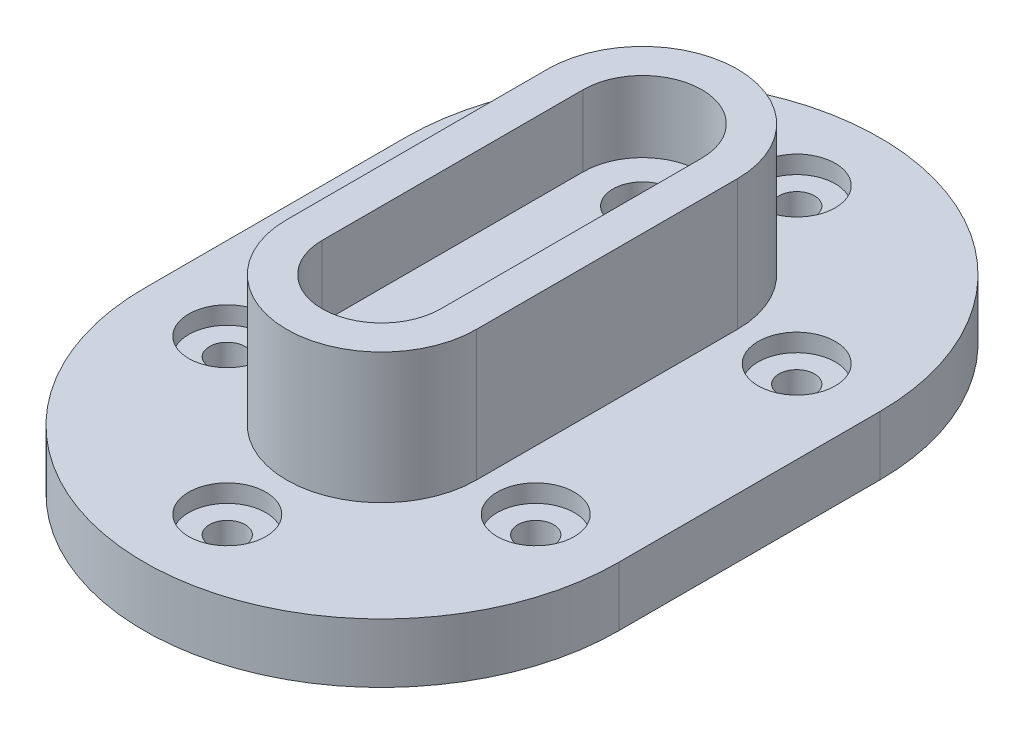
ISO-10303-21;
HEADER;
FILE_DESCRIPTION(('STEP AP214'),'2;1');
FILE_NAME('part.step','',(''),(''),'','','');
FILE_SCHEMA(('AUTOMOTIVE_DESIGN { 1 0 10303 214 1 1 1 1 }'));
ENDSEC;
DATA;
#1=APPLICATION_CONTEXT('core data for automotive mechanical design processes');
#2=APPLICATION_PROTOCOL_DEFINITION('international standard','automotive_design',2000,#1);
#3=PRODUCT_CONTEXT('',#1,'mechanical');
#4=PRODUCT('Part','Part','',(#3));
#5=PRODUCT_RELATED_PRODUCT_CATEGORY('part','',(#4));
#6=PRODUCT_DEFINITION_FORMATION('','',#4);
#7=PRODUCT_DEFINITION_CONTEXT('part definition',#1,'design');
#8=PRODUCT_DEFINITION('design','',#6,#7);
#9=PRODUCT_DEFINITION_SHAPE('','',#8);
#10=(LENGTH_UNIT() NAMED_UNIT(*) SI_UNIT(.MILLI.,.METRE.));
#11=(NAMED_UNIT(*) PLANE_ANGLE_UNIT() SI_UNIT($,.RADIAN.));
#12=(NAMED_UNIT(*) SI_UNIT($,.STERADIAN.) SOLID_ANGLE_UNIT());
#13=UNCERTAINTY_MEASURE_WITH_UNIT(LENGTH_MEASURE(1.E-05),#10,'distance_accuracy_value','');
#14=(GEOMETRIC_REPRESENTATION_CONTEXT(3) GLOBAL_UNCERTAINTY_ASSIGNED_CONTEXT((#13)) GLOBAL_UNIT_ASSIGNED_CONTEXT((#10,
#11,#12)) REPRESENTATION_CONTEXT('',''));
#15=CARTESIAN_POINT('',(0.,0.,0.));
#16=DIRECTION('',(0.,0.,1.));
#17=DIRECTION('',(1.,0.,0.));
#18=AXIS2_PLACEMENT_3D('',#15,#16,#17);
#19=CARTESIAN_POINT('',(0.,10.,-22.));
#20=DIRECTION('',(0.,1.,0.));
#21=DIRECTION('',(0.,0.,1.));
#22=AXIS2_PLACEMENT_3D('',#19,#20,#21);
#23=PLANE('',#22);
#24=CARTESIAN_POINT('',(0.,10.,48.));
#25=DIRECTION('',(0.,1.,0.));
#26=DIRECTION('',(0.,0.,1.));
#27=AXIS2_PLACEMENT_3D('',#24,#25,#26);
#28=CIRCLE('',#27,6.5);
#29=CARTESIAN_POINT('',(0.,10.,54.5));
#30=VERTEX_POINT('',#29);
#31=EDGE_CURVE('E272',#30,#30,#28,.T.);
#32=ORIENTED_EDGE('',*,*,#31,.F.);
#33=EDGE_LOOP('',(#32));
#34=FACE_BOUND('',#33,.T.);
#35=CARTESIAN_POINT('',(-26.,10.,-22.));
#36=DIRECTION('',(0.,1.,0.));
#37=DIRECTION('',(0.,0.,-1.));
#38=AXIS2_PLACEMENT_3D('',#35,#36,#37);
#39=CIRCLE('',#38,6.5);
#40=CARTESIAN_POINT('',(-26.,10.,-28.5));
#41=VERTEX_POINT('',#40);
#42=EDGE_CURVE('E270',#41,#41,#39,.T.);
#43=ORIENTED_EDGE('',*,*,#42,.F.);
#44=EDGE_LOOP('',(#43));
#45=FACE_BOUND('',#44,.T.);
#46=CARTESIAN_POINT('',(0.,10.,-48.));
#47=DIRECTION('',(0.,1.,0.));
#48=DIRECTION('',(0.,0.,1.));
#49=AXIS2_PLACEMENT_3D('',#46,#47,#48);
#50=CIRCLE('',#49,6.5);
#51=CARTESIAN_POINT('',(0.,10.,-41.5));
#52=VERTEX_POINT('',#51);
#53=EDGE_CURVE('E294',#52,#52,#50,.T.);
#54=ORIENTED_EDGE('',*,*,#53,.F.);
#55=EDGE_LOOP('',(#54));
#56=FACE_BOUND('',#55,.T.);
#57=CARTESIAN_POINT('',(26.,10.,22.));
#58=DIRECTION('',(0.,1.,0.));
#59=DIRECTION('',(0.,0.,1.));
#60=AXIS2_PLACEMENT_3D('',#57,#58,#59);
#61=CIRCLE('',#60,6.5);
#62=CARTESIAN_POINT('',(26.,10.,28.5));
#63=VERTEX_POINT('',#62);
#64=EDGE_CURVE('E281',#63,#63,#61,.T.);
#65=ORIENTED_EDGE('',*,*,#64,.F.);
#66=EDGE_LOOP('',(#65));
#67=FACE_BOUND('',#66,.T.);
#68=CARTESIAN_POINT('',(-26.,10.,22.));
#69=DIRECTION('',(0.,1.,0.));
#70=DIRECTION('',(0.,0.,1.));
#71=AXIS2_PLACEMENT_3D('',#68,#69,#70);
#72=CIRCLE('',#71,6.5);
#73=CARTESIAN_POINT('',(-26.,10.,28.5));
#74=VERTEX_POINT('',#73);
#75=EDGE_CURVE('E283',#74,#74,#72,.T.);
#76=ORIENTED_EDGE('',*,*,#75,.F.);
#77=EDGE_LOOP('',(#76));
#78=FACE_BOUND('',#77,.T.);
#79=CARTESIAN_POINT('',(26.,10.,-22.));
#80=DIRECTION('',(0.,1.,0.));
#81=DIRECTION('',(0.,0.,-1.));
#82=AXIS2_PLACEMENT_3D('',#79,#80,#81);
#83=CIRCLE('',#82,6.5);
#84=CARTESIAN_POINT('',(26.,10.,-28.5));
#85=VERTEX_POINT('',#84);
#86=EDGE_CURVE('E279',#85,#85,#83,.T.);
#87=ORIENTED_EDGE('',*,*,#86,.F.);
#88=EDGE_LOOP('',(#87));
#89=FACE_BOUND('',#88,.T.);
#90=CARTESIAN_POINT('',(0.,10.,-22.));
#91=DIRECTION('',(0.,1.,0.));
#92=DIRECTION('',(0.,0.,1.));
#93=AXIS2_PLACEMENT_3D('',#90,#91,#92);
#94=CIRCLE('',#93,40.);
#95=CARTESIAN_POINT('',(40.,10.,-22.));
#96=VERTEX_POINT('',#95);
#97=CARTESIAN_POINT('',(-40.,10.,-22.));
#98=VERTEX_POINT('',#97);
#99=EDGE_CURVE('E205',#96,#98,#94,.T.);
#100=ORIENTED_EDGE('',*,*,#99,.T.);
#101=DIRECTION('',(0.,0.,1.));
#102=VECTOR('',#101,1.);
#103=CARTESIAN_POINT('',(-40.,10.,-22.));
#104=LINE('',#103,#102);
#105=CARTESIAN_POINT('',(-40.,10.,22.));
#106=VERTEX_POINT('',#105);
#107=EDGE_CURVE('E207',#98,#106,#104,.T.);
#108=ORIENTED_EDGE('',*,*,#107,.T.);
#109=CARTESIAN_POINT('',(0.,10.,22.));
#110=DIRECTION('',(0.,1.,0.));
#111=DIRECTION('',(0.,0.,1.));
#112=AXIS2_PLACEMENT_3D('',#109,#110,#111);
#113=CIRCLE('',#112,40.);
#114=CARTESIAN_POINT('',(40.,10.,22.));
#115=VERTEX_POINT('',#114);
#116=EDGE_CURVE('E209',#106,#115,#113,.T.);
#117=ORIENTED_EDGE('',*,*,#116,.T.);
#118=DIRECTION('',(0.,0.,-1.));
#119=VECTOR('',#118,1.);
#120=CARTESIAN_POINT('',(40.,10.,-22.));
#121=LINE('',#120,#119);
#122=EDGE_CURVE('E212',#115,#96,#121,.T.);
#123=ORIENTED_EDGE('',*,*,#122,.T.);
#124=EDGE_LOOP('',(#100,#108,#117,#123));
#125=FACE_BOUND('',#124,.T.);
#126=DIRECTION('',(0.,0.,1.));
#127=VECTOR('',#126,1.);
#128=CARTESIAN_POINT('',(-16.,10.,-22.));
#129=LINE('',#128,#127);
#130=CARTESIAN_POINT('',(-16.,10.,-22.));
#131=VERTEX_POINT('',#130);
#132=CARTESIAN_POINT('',(-16.,10.,22.));
#133=VERTEX_POINT('',#132);
#134=EDGE_CURVE('E190',#131,#133,#129,.T.);
#135=ORIENTED_EDGE('',*,*,#134,.F.);
#136=CARTESIAN_POINT('',(0.,10.,-22.));
#137=DIRECTION('',(0.,1.,0.));
#138=DIRECTION('',(0.,0.,1.));
#139=AXIS2_PLACEMENT_3D('',#136,#137,#138);
#140=CIRCLE('',#139,16.);
#141=CARTESIAN_POINT('',(16.,10.,-22.));
#142=VERTEX_POINT('',#141);
#143=EDGE_CURVE('E173',#142,#131,#140,.T.);
#144=ORIENTED_EDGE('',*,*,#143,.F.);
#145=DIRECTION('',(0.,0.,-1.));
#146=VECTOR('',#145,1.);
#147=CARTESIAN_POINT('',(16.,10.,-22.));
#148=LINE('',#147,#146);
#149=CARTESIAN_POINT('',(16.,10.,22.));
#150=VERTEX_POINT('',#149);
#151=EDGE_CURVE('E178',#150,#142,#148,.T.);
#152=ORIENTED_EDGE('',*,*,#151,.F.);
#153=CARTESIAN_POINT('',(0.,10.,22.));
#154=DIRECTION('',(0.,1.,0.));
#155=DIRECTION('',(0.,0.,1.));
#156=AXIS2_PLACEMENT_3D('',#153,#154,#155);
#157=CIRCLE('',#156,16.);
#158=EDGE_CURVE('E186',#133,#150,#157,.T.);
#159=ORIENTED_EDGE('',*,*,#158,.F.);
#160=EDGE_LOOP('',(#135,#144,#152,#159));
#161=FACE_BOUND('',#160,.T.);
#162=ADVANCED_FACE('F44',(#34,#45,#56,#67,#78,#89,#125,#161),#23,.T.);
#163=CARTESIAN_POINT('',(0.,10.,-22.));
#164=DIRECTION('',(0.,-1.,0.));
#165=DIRECTION('',(0.,0.,-1.));
#166=AXIS2_PLACEMENT_3D('',#163,#164,#165);
#167=CYLINDRICAL_SURFACE('',#166,40.);
#168=CARTESIAN_POINT('',(0.,0.,-22.));
#169=DIRECTION('',(0.,1.,0.));
#170=DIRECTION('',(0.,0.,1.));
#171=AXIS2_PLACEMENT_3D('',#168,#169,#170);
#172=CIRCLE('',#171,40.);
#173=CARTESIAN_POINT('',(40.,0.,-22.));
#174=VERTEX_POINT('',#173);
#175=CARTESIAN_POINT('',(-40.,0.,-22.));
#176=VERTEX_POINT('',#175);
#177=EDGE_CURVE('E201',#174,#176,#172,.T.);
#178=ORIENTED_EDGE('',*,*,#177,.T.);
#179=DIRECTION('',(0.,-1.,0.));
#180=VECTOR('',#179,1.);
#181=CARTESIAN_POINT('',(-40.,10.,-22.));
#182=LINE('',#181,#180);
#183=EDGE_CURVE('E11',#98,#176,#182,.T.);
#184=ORIENTED_EDGE('',*,*,#183,.F.);
#185=ORIENTED_EDGE('',*,*,#99,.F.);
#186=DIRECTION('',(0.,-1.,0.));
#187=VECTOR('',#186,1.);
#188=CARTESIAN_POINT('',(40.,10.,-22.));
#189=LINE('',#188,#187);
#190=EDGE_CURVE('E214',#96,#174,#189,.T.);
#191=ORIENTED_EDGE('',*,*,#190,.T.);
#192=EDGE_LOOP('',(#178,#184,#185,#191));
#193=FACE_BOUND('',#192,.T.);
#194=ADVANCED_FACE('F50',(#193),#167,.T.);
#195=CARTESIAN_POINT('',(-40.,10.,-22.));
#196=DIRECTION('',(1.,0.,0.));
#197=DIRECTION('',(0.,0.,-1.));
#198=AXIS2_PLACEMENT_3D('',#195,#196,#197);
#199=PLANE('',#198);
#200=DIRECTION('',(0.,0.,1.));
#201=VECTOR('',#200,1.);
#202=CARTESIAN_POINT('',(-40.,0.,-22.));
#203=LINE('',#202,#201);
#204=CARTESIAN_POINT('',(-40.,0.,22.));
#205=VERTEX_POINT('',#204);
#206=EDGE_CURVE('E217',#176,#205,#203,.T.);
#207=ORIENTED_EDGE('',*,*,#206,.T.);
#208=DIRECTION('',(0.,-1.,0.));
#209=VECTOR('',#208,1.);
#210=CARTESIAN_POINT('',(-40.,10.,22.));
#211=LINE('',#210,#209);
#212=EDGE_CURVE('E53',#106,#205,#211,.T.);
#213=ORIENTED_EDGE('',*,*,#212,.F.);
#214=ORIENTED_EDGE('',*,*,#107,.F.);
#215=ORIENTED_EDGE('',*,*,#183,.T.);
#216=EDGE_LOOP('',(#207,#213,#214,#215));
#217=FACE_BOUND('',#216,.T.);
#218=ADVANCED_FACE('F335',(#217),#199,.F.);
#219=CARTESIAN_POINT('',(0.,10.,22.));
#220=DIRECTION('',(0.,-1.,0.));
#221=DIRECTION('',(0.,0.,-1.));
#222=AXIS2_PLACEMENT_3D('',#219,#220,#221);
#223=CYLINDRICAL_SURFACE('',#222,40.);
#224=CARTESIAN_POINT('',(0.,0.,22.));
#225=DIRECTION('',(0.,1.,0.));
#226=DIRECTION('',(0.,0.,1.));
#227=AXIS2_PLACEMENT_3D('',#224,#225,#226);
#228=CIRCLE('',#227,40.);
#229=CARTESIAN_POINT('',(40.,0.,22.));
#230=VERTEX_POINT('',#229);
#231=EDGE_CURVE('E219',#205,#230,#228,.T.);
#232=ORIENTED_EDGE('',*,*,#231,.T.);
#233=DIRECTION('',(0.,-1.,0.));
#234=VECTOR('',#233,1.);
#235=CARTESIAN_POINT('',(40.,10.,22.));
#236=LINE('',#235,#234);
#237=EDGE_CURVE('E225',#115,#230,#236,.T.);
#238=ORIENTED_EDGE('',*,*,#237,.F.);
#239=ORIENTED_EDGE('',*,*,#116,.F.);
#240=ORIENTED_EDGE('',*,*,#212,.T.);
#241=EDGE_LOOP('',(#232,#238,#239,#240));
#242=FACE_BOUND('',#241,.T.);
#243=ADVANCED_FACE('F349',(#242),#223,.T.);
#244=CARTESIAN_POINT('',(40.,10.,-22.));
#245=DIRECTION('',(-1.,0.,0.));
#246=DIRECTION('',(0.,0.,1.));
#247=AXIS2_PLACEMENT_3D('',#244,#245,#246);
#248=PLANE('',#247);
#249=DIRECTION('',(0.,0.,-1.));
#250=VECTOR('',#249,1.);
#251=CARTESIAN_POINT('',(40.,0.,-22.));
#252=LINE('',#251,#250);
#253=EDGE_CURVE('E210',#230,#174,#252,.T.);
#254=ORIENTED_EDGE('',*,*,#253,.T.);
#255=ORIENTED_EDGE('',*,*,#190,.F.);
#256=ORIENTED_EDGE('',*,*,#122,.F.);
#257=ORIENTED_EDGE('',*,*,#237,.T.);
#258=EDGE_LOOP('',(#254,#255,#256,#257));
#259=FACE_BOUND('',#258,.T.);
#260=ADVANCED_FACE('F341',(#259),#248,.F.);
#261=CARTESIAN_POINT('',(0.,0.,-22.));
#262=DIRECTION('',(0.,1.,0.));
#263=DIRECTION('',(0.,0.,1.));
#264=AXIS2_PLACEMENT_3D('',#261,#262,#263);
#265=PLANE('',#264);
#266=CARTESIAN_POINT('',(0.,0.,48.));
#267=DIRECTION('',(0.,1.,0.));
#268=DIRECTION('',(0.,0.,1.));
#269=AXIS2_PLACEMENT_3D('',#266,#267,#268);
#270=CIRCLE('',#269,3.);
#271=CARTESIAN_POINT('',(0.,0.,51.));
#272=VERTEX_POINT('',#271);
#273=EDGE_CURVE('E237',#272,#272,#270,.T.);
#274=ORIENTED_EDGE('',*,*,#273,.T.);
#275=EDGE_LOOP('',(#274));
#276=FACE_BOUND('',#275,.T.);
#277=CARTESIAN_POINT('',(-26.,0.,22.));
#278=DIRECTION('',(0.,1.,0.));
#279=DIRECTION('',(0.,0.,1.));
#280=AXIS2_PLACEMENT_3D('',#277,#278,#279);
#281=CIRCLE('',#280,3.);
#282=CARTESIAN_POINT('',(-26.,0.,25.));
#283=VERTEX_POINT('',#282);
#284=EDGE_CURVE('E254',#283,#283,#281,.T.);
#285=ORIENTED_EDGE('',*,*,#284,.T.);
#286=EDGE_LOOP('',(#285));
#287=FACE_BOUND('',#286,.T.);
#288=CARTESIAN_POINT('',(-26.,0.,-22.));
#289=DIRECTION('',(0.,1.,0.));
#290=DIRECTION('',(0.,0.,1.));
#291=AXIS2_PLACEMENT_3D('',#288,#289,#290);
#292=CIRCLE('',#291,3.);
#293=CARTESIAN_POINT('',(-26.,0.,-19.));
#294=VERTEX_POINT('',#293);
#295=EDGE_CURVE('E243',#294,#294,#292,.T.);
#296=ORIENTED_EDGE('',*,*,#295,.T.);
#297=EDGE_LOOP('',(#296));
#298=FACE_BOUND('',#297,.T.);
#299=CARTESIAN_POINT('',(0.,0.,-48.));
#300=DIRECTION('',(0.,1.,0.));
#301=DIRECTION('',(0.,0.,1.));
#302=AXIS2_PLACEMENT_3D('',#299,#300,#301);
#303=CIRCLE('',#302,3.);
#304=CARTESIAN_POINT('',(0.,0.,-45.));
#305=VERTEX_POINT('',#304);
#306=EDGE_CURVE('E250',#305,#305,#303,.T.);
#307=ORIENTED_EDGE('',*,*,#306,.T.);
#308=EDGE_LOOP('',(#307));
#309=FACE_BOUND('',#308,.T.);
#310=CARTESIAN_POINT('',(26.,0.,-22.));
#311=DIRECTION('',(0.,1.,0.));
#312=DIRECTION('',(0.,0.,1.));
#313=AXIS2_PLACEMENT_3D('',#310,#311,#312);
#314=CIRCLE('',#313,3.);
#315=CARTESIAN_POINT('',(26.,0.,-19.));
#316=VERTEX_POINT('',#315);
#317=EDGE_CURVE('E263',#316,#316,#314,.T.);
#318=ORIENTED_EDGE('',*,*,#317,.T.);
#319=EDGE_LOOP('',(#318));
#320=FACE_BOUND('',#319,.T.);
#321=CARTESIAN_POINT('',(26.,0.,22.));
#322=DIRECTION('',(0.,1.,0.));
#323=DIRECTION('',(0.,0.,1.));
#324=AXIS2_PLACEMENT_3D('',#321,#322,#323);
#325=CIRCLE('',#324,3.);
#326=CARTESIAN_POINT('',(26.,0.,25.));
#327=VERTEX_POINT('',#326);
#328=EDGE_CURVE('E249',#327,#327,#325,.T.);
#329=ORIENTED_EDGE('',*,*,#328,.T.);
#330=EDGE_LOOP('',(#329));
#331=FACE_BOUND('',#330,.T.);
#332=CARTESIAN_POINT('',(0.,0.,-22.));
#333=DIRECTION('',(0.,1.,0.));
#334=DIRECTION('',(0.,0.,1.));
#335=AXIS2_PLACEMENT_3D('',#332,#333,#334);
#336=CIRCLE('',#335,5.);
#337=CARTESIAN_POINT('',(0.,0.,-17.));
#338=VERTEX_POINT('',#337);
#339=EDGE_CURVE('E151',#338,#338,#336,.T.);
#340=ORIENTED_EDGE('',*,*,#339,.T.);
#341=EDGE_LOOP('',(#340));
#342=FACE_BOUND('',#341,.T.);
#343=CARTESIAN_POINT('',(0.,0.,22.));
#344=DIRECTION('',(0.,1.,0.));
#345=DIRECTION('',(0.,0.,1.));
#346=AXIS2_PLACEMENT_3D('',#343,#344,#345);
#347=CIRCLE('',#346,5.);
#348=CARTESIAN_POINT('',(0.,0.,27.));
#349=VERTEX_POINT('',#348);
#350=EDGE_CURVE('E233',#349,#349,#347,.T.);
#351=ORIENTED_EDGE('',*,*,#350,.T.);
#352=EDGE_LOOP('',(#351));
#353=FACE_BOUND('',#352,.T.);
#354=ORIENTED_EDGE('',*,*,#177,.F.);
#355=ORIENTED_EDGE('',*,*,#253,.F.);
#356=ORIENTED_EDGE('',*,*,#231,.F.);
#357=ORIENTED_EDGE('',*,*,#206,.F.);
#358=EDGE_LOOP('',(#354,#355,#356,#357));
#359=FACE_BOUND('',#358,.T.);
#360=ADVANCED_FACE('F308',(#276,#287,#298,#309,#320,#331,#342,#353,#359),#265,.F.);
#361=CARTESIAN_POINT('',(0.,32.,-22.));
#362=DIRECTION('',(0.,1.,0.));
#363=DIRECTION('',(0.,0.,1.));
#364=AXIS2_PLACEMENT_3D('',#361,#362,#363);
#365=PLANE('',#364);
#366=CARTESIAN_POINT('',(0.,32.,-22.));
#367=DIRECTION('',(0.,1.,0.));
#368=DIRECTION('',(0.,0.,1.));
#369=AXIS2_PLACEMENT_3D('',#366,#367,#368);
#370=CIRCLE('',#369,16.);
#371=CARTESIAN_POINT('',(16.,32.,-22.));
#372=VERTEX_POINT('',#371);
#373=CARTESIAN_POINT('',(-16.,32.,-22.));
#374=VERTEX_POINT('',#373);
#375=EDGE_CURVE('E172',#372,#374,#370,.T.);
#376=ORIENTED_EDGE('',*,*,#375,.T.);
#377=DIRECTION('',(0.,0.,1.));
#378=VECTOR('',#377,1.);
#379=CARTESIAN_POINT('',(-16.,32.,-22.));
#380=LINE('',#379,#378);
#381=CARTESIAN_POINT('',(-16.,32.,22.));
#382=VERTEX_POINT('',#381);
#383=EDGE_CURVE('E180',#374,#382,#380,.T.);
#384=ORIENTED_EDGE('',*,*,#383,.T.);
#385=CARTESIAN_POINT('',(0.,32.,22.));
#386=DIRECTION('',(0.,1.,0.));
#387=DIRECTION('',(0.,0.,1.));
#388=AXIS2_PLACEMENT_3D('',#385,#386,#387);
#389=CIRCLE('',#388,16.);
#390=CARTESIAN_POINT('',(16.,32.,22.));
#391=VERTEX_POINT('',#390);
#392=EDGE_CURVE('E179',#382,#391,#389,.T.);
#393=ORIENTED_EDGE('',*,*,#392,.T.);
#394=DIRECTION('',(0.,0.,-1.));
#395=VECTOR('',#394,1.);
#396=CARTESIAN_POINT('',(16.,32.,-22.));
#397=LINE('',#396,#395);
#398=EDGE_CURVE('E185',#391,#372,#397,.T.);
#399=ORIENTED_EDGE('',*,*,#398,.T.);
#400=EDGE_LOOP('',(#376,#384,#393,#399));
#401=FACE_BOUND('',#400,.T.);
#402=DIRECTION('',(0.,0.,1.));
#403=VECTOR('',#402,1.);
#404=CARTESIAN_POINT('',(-10.,32.,-22.));
#405=LINE('',#404,#403);
#406=CARTESIAN_POINT('',(-10.,32.,-22.));
#407=VERTEX_POINT('',#406);
#408=CARTESIAN_POINT('',(-10.,32.,22.));
#409=VERTEX_POINT('',#408);
#410=EDGE_CURVE('E158',#407,#409,#405,.T.);
#411=ORIENTED_EDGE('',*,*,#410,.F.);
#412=CARTESIAN_POINT('',(0.,32.,-22.));
#413=DIRECTION('',(0.,1.,0.));
#414=DIRECTION('',(0.,0.,1.));
#415=AXIS2_PLACEMENT_3D('',#412,#413,#414);
#416=CIRCLE('',#415,10.);
#417=CARTESIAN_POINT('',(10.,32.,-22.));
#418=VERTEX_POINT('',#417);
#419=EDGE_CURVE('E156',#418,#407,#416,.T.);
#420=ORIENTED_EDGE('',*,*,#419,.F.);
#421=DIRECTION('',(0.,0.,-1.));
#422=VECTOR('',#421,1.);
#423=CARTESIAN_POINT('',(10.,32.,-22.));
#424=LINE('',#423,#422);
#425=CARTESIAN_POINT('',(10.,32.,22.));
#426=VERTEX_POINT('',#425);
#427=EDGE_CURVE('E144',#426,#418,#424,.T.);
#428=ORIENTED_EDGE('',*,*,#427,.F.);
#429=CARTESIAN_POINT('',(0.,32.,22.));
#430=DIRECTION('',(0.,1.,0.));
#431=DIRECTION('',(0.,0.,1.));
#432=AXIS2_PLACEMENT_3D('',#429,#430,#431);
#433=CIRCLE('',#432,10.);
#434=EDGE_CURVE('E164',#409,#426,#433,.T.);
#435=ORIENTED_EDGE('',*,*,#434,.F.);
#436=EDGE_LOOP('',(#411,#420,#428,#435));
#437=FACE_BOUND('',#436,.T.);
#438=ADVANCED_FACE('F344',(#401,#437),#365,.T.);
#439=CARTESIAN_POINT('',(0.,32.,-22.));
#440=DIRECTION('',(0.,-1.,0.));
#441=DIRECTION('',(0.,0.,-1.));
#442=AXIS2_PLACEMENT_3D('',#439,#440,#441);
#443=CYLINDRICAL_SURFACE('',#442,16.);
#444=ORIENTED_EDGE('',*,*,#143,.T.);
#445=DIRECTION('',(0.,-1.,0.));
#446=VECTOR('',#445,1.);
#447=CARTESIAN_POINT('',(-16.,32.,-22.));
#448=LINE('',#447,#446);
#449=EDGE_CURVE('E198',#374,#131,#448,.T.);
#450=ORIENTED_EDGE('',*,*,#449,.F.);
#451=ORIENTED_EDGE('',*,*,#375,.F.);
#452=DIRECTION('',(0.,-1.,0.));
#453=VECTOR('',#452,1.);
#454=CARTESIAN_POINT('',(16.,32.,-22.));
#455=LINE('',#454,#453);
#456=EDGE_CURVE('E183',#372,#142,#455,.T.);
#457=ORIENTED_EDGE('',*,*,#456,.T.);
#458=EDGE_LOOP('',(#444,#450,#451,#457));
#459=FACE_BOUND('',#458,.T.);
#460=ADVANCED_FACE('F339',(#459),#443,.T.);
#461=CARTESIAN_POINT('',(-16.,32.,-22.));
#462=DIRECTION('',(1.,0.,0.));
#463=DIRECTION('',(0.,0.,-1.));
#464=AXIS2_PLACEMENT_3D('',#461,#462,#463);
#465=PLANE('',#464);
#466=ORIENTED_EDGE('',*,*,#134,.T.);
#467=DIRECTION('',(0.,-1.,0.));
#468=VECTOR('',#467,1.);
#469=CARTESIAN_POINT('',(-16.,32.,22.));
#470=LINE('',#469,#468);
#471=EDGE_CURVE('E200',#382,#133,#470,.T.);
#472=ORIENTED_EDGE('',*,*,#471,.F.);
#473=ORIENTED_EDGE('',*,*,#383,.F.);
#474=ORIENTED_EDGE('',*,*,#449,.T.);
#475=EDGE_LOOP('',(#466,#472,#473,#474));
#476=FACE_BOUND('',#475,.T.);
#477=ADVANCED_FACE('F374',(#476),#465,.F.);
#478=CARTESIAN_POINT('',(0.,32.,22.));
#479=DIRECTION('',(0.,-1.,0.));
#480=DIRECTION('',(0.,0.,-1.));
#481=AXIS2_PLACEMENT_3D('',#478,#479,#480);
#482=CYLINDRICAL_SURFACE('',#481,16.);
#483=ORIENTED_EDGE('',*,*,#158,.T.);
#484=DIRECTION('',(0.,-1.,0.));
#485=VECTOR('',#484,1.);
#486=CARTESIAN_POINT('',(16.,32.,22.));
#487=LINE('',#486,#485);
#488=EDGE_CURVE('E193',#391,#150,#487,.T.);
#489=ORIENTED_EDGE('',*,*,#488,.F.);
#490=ORIENTED_EDGE('',*,*,#392,.F.);
#491=ORIENTED_EDGE('',*,*,#471,.T.);
#492=EDGE_LOOP('',(#483,#489,#490,#491));
#493=FACE_BOUND('',#492,.T.);
#494=ADVANCED_FACE('F378',(#493),#482,.T.);
#495=CARTESIAN_POINT('',(16.,32.,-22.));
#496=DIRECTION('',(-1.,0.,0.));
#497=DIRECTION('',(0.,0.,1.));
#498=AXIS2_PLACEMENT_3D('',#495,#496,#497);
#499=PLANE('',#498);
#500=ORIENTED_EDGE('',*,*,#151,.T.);
#501=ORIENTED_EDGE('',*,*,#456,.F.);
#502=ORIENTED_EDGE('',*,*,#398,.F.);
#503=ORIENTED_EDGE('',*,*,#488,.T.);
#504=EDGE_LOOP('',(#500,#501,#502,#503));
#505=FACE_BOUND('',#504,.T.);
#506=ADVANCED_FACE('F389',(#505),#499,.F.);
#507=CARTESIAN_POINT('',(0.,32.,-22.));
#508=DIRECTION('',(0.,-1.,0.));
#509=DIRECTION('',(0.,0.,-1.));
#510=AXIS2_PLACEMENT_3D('',#507,#508,#509);
#511=CYLINDRICAL_SURFACE('',#510,10.);
#512=CARTESIAN_POINT('',(0.,20.,-22.));
#513=DIRECTION('',(0.,1.,0.));
#514=DIRECTION('',(0.,0.,1.));
#515=AXIS2_PLACEMENT_3D('',#512,#513,#514);
#516=CIRCLE('',#515,10.);
#517=CARTESIAN_POINT('',(10.,20.,-22.));
#518=VERTEX_POINT('',#517);
#519=CARTESIAN_POINT('',(-10.,20.,-22.));
#520=VERTEX_POINT('',#519);
#521=EDGE_CURVE('E148',#518,#520,#516,.T.);
#522=ORIENTED_EDGE('',*,*,#521,.F.);
#523=DIRECTION('',(0.,-1.,0.));
#524=VECTOR('',#523,1.);
#525=CARTESIAN_POINT('',(10.,32.,-22.));
#526=LINE('',#525,#524);
#527=EDGE_CURVE('E140',#418,#518,#526,.T.);
#528=ORIENTED_EDGE('',*,*,#527,.F.);
#529=ORIENTED_EDGE('',*,*,#419,.T.);
#530=DIRECTION('',(0.,-1.,0.));
#531=VECTOR('',#530,1.);
#532=CARTESIAN_POINT('',(-10.,32.,-22.));
#533=LINE('',#532,#531);
#534=EDGE_CURVE('E155',#407,#520,#533,.T.);
#535=ORIENTED_EDGE('',*,*,#534,.T.);
#536=EDGE_LOOP('',(#522,#528,#529,#535));
#537=FACE_BOUND('',#536,.T.);
#538=ADVANCED_FACE('F152',(#537),#511,.F.);
#539=CARTESIAN_POINT('',(-10.,32.,-22.));
#540=DIRECTION('',(1.,0.,0.));
#541=DIRECTION('',(0.,0.,-1.));
#542=AXIS2_PLACEMENT_3D('',#539,#540,#541);
#543=PLANE('',#542);
#544=DIRECTION('',(0.,0.,1.));
#545=VECTOR('',#544,1.);
#546=CARTESIAN_POINT('',(-10.,20.,-22.));
#547=LINE('',#546,#545);
#548=CARTESIAN_POINT('',(-10.,20.,22.));
#549=VERTEX_POINT('',#548);
#550=EDGE_CURVE('E65',#520,#549,#547,.T.);
#551=ORIENTED_EDGE('',*,*,#550,.F.);
#552=ORIENTED_EDGE('',*,*,#534,.F.);
#553=ORIENTED_EDGE('',*,*,#410,.T.);
#554=DIRECTION('',(0.,-1.,0.));
#555=VECTOR('',#554,1.);
#556=CARTESIAN_POINT('',(-10.,32.,22.));
#557=LINE('',#556,#555);
#558=EDGE_CURVE('E167',#409,#549,#557,.T.);
#559=ORIENTED_EDGE('',*,*,#558,.T.);
#560=EDGE_LOOP('',(#551,#552,#553,#559));
#561=FACE_BOUND('',#560,.T.);
#562=ADVANCED_FACE('F393',(#561),#543,.T.);
#563=CARTESIAN_POINT('',(0.,32.,22.));
#564=DIRECTION('',(0.,-1.,0.));
#565=DIRECTION('',(0.,0.,-1.));
#566=AXIS2_PLACEMENT_3D('',#563,#564,#565);
#567=CYLINDRICAL_SURFACE('',#566,10.);
#568=CARTESIAN_POINT('',(0.,20.,22.));
#569=DIRECTION('',(0.,1.,0.));
#570=DIRECTION('',(0.,0.,1.));
#571=AXIS2_PLACEMENT_3D('',#568,#569,#570);
#572=CIRCLE('',#571,10.);
#573=CARTESIAN_POINT('',(10.,20.,22.));
#574=VERTEX_POINT('',#573);
#575=EDGE_CURVE('E68',#549,#574,#572,.T.);
#576=ORIENTED_EDGE('',*,*,#575,.F.);
#577=ORIENTED_EDGE('',*,*,#558,.F.);
#578=ORIENTED_EDGE('',*,*,#434,.T.);
#579=DIRECTION('',(0.,-1.,0.));
#580=VECTOR('',#579,1.);
#581=CARTESIAN_POINT('',(10.,32.,22.));
#582=LINE('',#581,#580);
#583=EDGE_CURVE('E150',#426,#574,#582,.T.);
#584=ORIENTED_EDGE('',*,*,#583,.T.);
#585=EDGE_LOOP('',(#576,#577,#578,#584));
#586=FACE_BOUND('',#585,.T.);
#587=ADVANCED_FACE('F736',(#586),#567,.F.);
#588=CARTESIAN_POINT('',(10.,32.,-22.));
#589=DIRECTION('',(-1.,0.,0.));
#590=DIRECTION('',(0.,0.,1.));
#591=AXIS2_PLACEMENT_3D('',#588,#589,#590);
#592=PLANE('',#591);
#593=DIRECTION('',(0.,0.,-1.));
#594=VECTOR('',#593,1.);
#595=CARTESIAN_POINT('',(10.,20.,22.));
#596=LINE('',#595,#594);
#597=EDGE_CURVE('E145',#574,#518,#596,.T.);
#598=ORIENTED_EDGE('',*,*,#597,.F.);
#599=ORIENTED_EDGE('',*,*,#583,.F.);
#600=ORIENTED_EDGE('',*,*,#427,.T.);
#601=ORIENTED_EDGE('',*,*,#527,.T.);
#602=EDGE_LOOP('',(#598,#599,#600,#601));
#603=FACE_BOUND('',#602,.T.);
#604=ADVANCED_FACE('F137',(#603),#592,.T.);
#605=CARTESIAN_POINT('',(0.,20.,-22.));
#606=DIRECTION('',(0.,1.,0.));
#607=DIRECTION('',(0.,0.,1.));
#608=AXIS2_PLACEMENT_3D('',#605,#606,#607);
#609=PLANE('',#608);
#610=CARTESIAN_POINT('',(0.,20.,-22.));
#611=DIRECTION('',(0.,1.,0.));
#612=DIRECTION('',(0.,0.,1.));
#613=AXIS2_PLACEMENT_3D('',#610,#611,#612);
#614=CIRCLE('',#613,5.);
#615=CARTESIAN_POINT('',(0.,20.,-17.));
#616=VERTEX_POINT('',#615);
#617=EDGE_CURVE('E231',#616,#616,#614,.T.);
#618=ORIENTED_EDGE('',*,*,#617,.F.);
#619=EDGE_LOOP('',(#618));
#620=FACE_BOUND('',#619,.T.);
#621=CARTESIAN_POINT('',(0.,20.,22.));
#622=DIRECTION('',(0.,1.,0.));
#623=DIRECTION('',(0.,0.,1.));
#624=AXIS2_PLACEMENT_3D('',#621,#622,#623);
#625=CIRCLE('',#624,5.);
#626=CARTESIAN_POINT('',(0.,20.,27.));
#627=VERTEX_POINT('',#626);
#628=EDGE_CURVE('E226',#627,#627,#625,.T.);
#629=ORIENTED_EDGE('',*,*,#628,.F.);
#630=EDGE_LOOP('',(#629));
#631=FACE_BOUND('',#630,.T.);
#632=ORIENTED_EDGE('',*,*,#521,.T.);
#633=ORIENTED_EDGE('',*,*,#550,.T.);
#634=ORIENTED_EDGE('',*,*,#575,.T.);
#635=ORIENTED_EDGE('',*,*,#597,.T.);
#636=EDGE_LOOP('',(#632,#633,#634,#635));
#637=FACE_BOUND('',#636,.T.);
#638=ADVANCED_FACE('F159',(#620,#631,#637),#609,.T.);
#639=CARTESIAN_POINT('',(0.,-24.5,22.));
#640=DIRECTION('',(0.,1.,0.));
#641=DIRECTION('',(0.,0.,1.));
#642=AXIS2_PLACEMENT_3D('',#639,#640,#641);
#643=CYLINDRICAL_SURFACE('',#642,5.);
#644=ORIENTED_EDGE('',*,*,#628,.T.);
#645=EDGE_LOOP('',(#644));
#646=FACE_BOUND('',#645,.T.);
#647=ORIENTED_EDGE('',*,*,#350,.F.);
#648=EDGE_LOOP('',(#647));
#649=FACE_BOUND('',#648,.T.);
#650=ADVANCED_FACE('F313',(#646,#649),#643,.F.);
#651=CARTESIAN_POINT('',(0.,-24.5,-22.));
#652=DIRECTION('',(0.,1.,0.));
#653=DIRECTION('',(0.,0.,1.));
#654=AXIS2_PLACEMENT_3D('',#651,#652,#653);
#655=CYLINDRICAL_SURFACE('',#654,5.);
#656=ORIENTED_EDGE('',*,*,#617,.T.);
#657=EDGE_LOOP('',(#656));
#658=FACE_BOUND('',#657,.T.);
#659=ORIENTED_EDGE('',*,*,#339,.F.);
#660=EDGE_LOOP('',(#659));
#661=FACE_BOUND('',#660,.T.);
#662=ADVANCED_FACE('F311',(#658,#661),#655,.F.);
#663=CARTESIAN_POINT('',(26.,7.,-22.));
#664=DIRECTION('',(0.,1.,0.));
#665=DIRECTION('',(0.,0.,1.));
#666=AXIS2_PLACEMENT_3D('',#663,#664,#665);
#667=CYLINDRICAL_SURFACE('',#666,6.5);
#668=CARTESIAN_POINT('',(26.,7.,-22.));
#669=DIRECTION('',(0.,1.,0.));
#670=DIRECTION('',(0.,0.,-1.));
#671=AXIS2_PLACEMENT_3D('',#668,#669,#670);
#672=CIRCLE('',#671,6.5);
#673=CARTESIAN_POINT('',(26.,7.,-28.5));
#674=VERTEX_POINT('',#673);
#675=EDGE_CURVE('E290',#674,#674,#672,.T.);
#676=ORIENTED_EDGE('',*,*,#675,.F.);
#677=EDGE_LOOP('',(#676));
#678=FACE_BOUND('',#677,.T.);
#679=ORIENTED_EDGE('',*,*,#86,.T.);
#680=EDGE_LOOP('',(#679));
#681=FACE_BOUND('',#680,.T.);
#682=ADVANCED_FACE('F312',(#678,#681),#667,.F.);
#683=CARTESIAN_POINT('',(26.,7.,-22.));
#684=DIRECTION('',(0.,-1.,0.));
#685=DIRECTION('',(0.,0.,-1.));
#686=AXIS2_PLACEMENT_3D('',#683,#684,#685);
#687=PLANE('',#686);
#688=CARTESIAN_POINT('',(26.,7.00000000000001,-22.));
#689=DIRECTION('',(0.,-1.,0.));
#690=DIRECTION('',(0.,0.,-1.));
#691=AXIS2_PLACEMENT_3D('',#688,#689,#690);
#692=CIRCLE('',#691,3.);
#693=CARTESIAN_POINT('',(26.,7.00000000000001,-25.));
#694=VERTEX_POINT('',#693);
#695=EDGE_CURVE('E47',#694,#694,#692,.T.);
#696=ORIENTED_EDGE('',*,*,#695,.T.);
#697=EDGE_LOOP('',(#696));
#698=FACE_BOUND('',#697,.T.);
#699=ORIENTED_EDGE('',*,*,#675,.T.);
#700=EDGE_LOOP('',(#699));
#701=FACE_BOUND('',#700,.T.);
#702=ADVANCED_FACE('F322',(#698,#701),#687,.F.);
#703=CARTESIAN_POINT('',(-26.,7.,22.));
#704=DIRECTION('',(0.,1.,0.));
#705=DIRECTION('',(0.,0.,1.));
#706=AXIS2_PLACEMENT_3D('',#703,#704,#705);
#707=CYLINDRICAL_SURFACE('',#706,6.5);
#708=CARTESIAN_POINT('',(-26.,7.,22.));
#709=DIRECTION('',(0.,1.,0.));
#710=DIRECTION('',(0.,0.,1.));
#711=AXIS2_PLACEMENT_3D('',#708,#709,#710);
#712=CIRCLE('',#711,6.5);
#713=CARTESIAN_POINT('',(-26.,7.,28.5));
#714=VERTEX_POINT('',#713);
#715=EDGE_CURVE('E282',#714,#714,#712,.T.);
#716=ORIENTED_EDGE('',*,*,#715,.F.);
#717=EDGE_LOOP('',(#716));
#718=FACE_BOUND('',#717,.T.);
#719=ORIENTED_EDGE('',*,*,#75,.T.);
#720=EDGE_LOOP('',(#719));
#721=FACE_BOUND('',#720,.T.);
#722=ADVANCED_FACE('F456',(#718,#721),#707,.F.);
#723=CARTESIAN_POINT('',(-26.,7.,22.));
#724=DIRECTION('',(0.,1.,0.));
#725=DIRECTION('',(0.,0.,1.));
#726=AXIS2_PLACEMENT_3D('',#723,#724,#725);
#727=PLANE('',#726);
#728=CARTESIAN_POINT('',(-26.,7.00000000000001,22.));
#729=DIRECTION('',(0.,1.,0.));
#730=DIRECTION('',(0.,0.,1.));
#731=AXIS2_PLACEMENT_3D('',#728,#729,#730);
#732=CIRCLE('',#731,3.);
#733=CARTESIAN_POINT('',(-26.,7.00000000000001,25.));
#734=VERTEX_POINT('',#733);
#735=EDGE_CURVE('E252',#734,#734,#732,.T.);
#736=ORIENTED_EDGE('',*,*,#735,.F.);
#737=EDGE_LOOP('',(#736));
#738=FACE_BOUND('',#737,.T.);
#739=ORIENTED_EDGE('',*,*,#715,.T.);
#740=EDGE_LOOP('',(#739));
#741=FACE_BOUND('',#740,.T.);
#742=ADVANCED_FACE('F462',(#738,#741),#727,.T.);
#743=CARTESIAN_POINT('',(26.,7.,22.));
#744=DIRECTION('',(0.,1.,0.));
#745=DIRECTION('',(0.,0.,1.));
#746=AXIS2_PLACEMENT_3D('',#743,#744,#745);
#747=CYLINDRICAL_SURFACE('',#746,6.5);
#748=CARTESIAN_POINT('',(26.,7.,22.));
#749=DIRECTION('',(0.,1.,0.));
#750=DIRECTION('',(0.,0.,1.));
#751=AXIS2_PLACEMENT_3D('',#748,#749,#750);
#752=CIRCLE('',#751,6.5);
#753=CARTESIAN_POINT('',(26.,7.,28.5));
#754=VERTEX_POINT('',#753);
#755=EDGE_CURVE('E296',#754,#754,#752,.T.);
#756=ORIENTED_EDGE('',*,*,#755,.F.);
#757=EDGE_LOOP('',(#756));
#758=FACE_BOUND('',#757,.T.);
#759=ORIENTED_EDGE('',*,*,#64,.T.);
#760=EDGE_LOOP('',(#759));
#761=FACE_BOUND('',#760,.T.);
#762=ADVANCED_FACE('F477',(#758,#761),#747,.F.);
#763=CARTESIAN_POINT('',(26.,7.,22.));
#764=DIRECTION('',(0.,1.,0.));
#765=DIRECTION('',(0.,0.,1.));
#766=AXIS2_PLACEMENT_3D('',#763,#764,#765);
#767=PLANE('',#766);
#768=CARTESIAN_POINT('',(26.,7.00000000000001,22.));
#769=DIRECTION('',(0.,1.,0.));
#770=DIRECTION('',(0.,0.,1.));
#771=AXIS2_PLACEMENT_3D('',#768,#769,#770);
#772=CIRCLE('',#771,3.);
#773=CARTESIAN_POINT('',(26.,7.00000000000001,25.));
#774=VERTEX_POINT('',#773);
#775=EDGE_CURVE('E247',#774,#774,#772,.T.);
#776=ORIENTED_EDGE('',*,*,#775,.F.);
#777=EDGE_LOOP('',(#776));
#778=FACE_BOUND('',#777,.T.);
#779=ORIENTED_EDGE('',*,*,#755,.T.);
#780=EDGE_LOOP('',(#779));
#781=FACE_BOUND('',#780,.T.);
#782=ADVANCED_FACE('F484',(#778,#781),#767,.T.);
#783=CARTESIAN_POINT('',(0.,7.,-48.));
#784=DIRECTION('',(0.,1.,0.));
#785=DIRECTION('',(0.,0.,1.));
#786=AXIS2_PLACEMENT_3D('',#783,#784,#785);
#787=CYLINDRICAL_SURFACE('',#786,6.5);
#788=CARTESIAN_POINT('',(0.,7.,-48.));
#789=DIRECTION('',(0.,1.,0.));
#790=DIRECTION('',(0.,0.,1.));
#791=AXIS2_PLACEMENT_3D('',#788,#789,#790);
#792=CIRCLE('',#791,6.5);
#793=CARTESIAN_POINT('',(0.,7.,-41.5));
#794=VERTEX_POINT('',#793);
#795=EDGE_CURVE('E274',#794,#794,#792,.T.);
#796=ORIENTED_EDGE('',*,*,#795,.F.);
#797=EDGE_LOOP('',(#796));
#798=FACE_BOUND('',#797,.T.);
#799=ORIENTED_EDGE('',*,*,#53,.T.);
#800=EDGE_LOOP('',(#799));
#801=FACE_BOUND('',#800,.T.);
#802=ADVANCED_FACE('F490',(#798,#801),#787,.F.);
#803=CARTESIAN_POINT('',(0.,7.,-48.));
#804=DIRECTION('',(0.,1.,0.));
#805=DIRECTION('',(0.,0.,1.));
#806=AXIS2_PLACEMENT_3D('',#803,#804,#805);
#807=PLANE('',#806);
#808=CARTESIAN_POINT('',(0.,7.00000000000001,-48.));
#809=DIRECTION('',(0.,1.,0.));
#810=DIRECTION('',(0.,0.,1.));
#811=AXIS2_PLACEMENT_3D('',#808,#809,#810);
#812=CIRCLE('',#811,3.);
#813=CARTESIAN_POINT('',(0.,7.00000000000001,-45.));
#814=VERTEX_POINT('',#813);
#815=EDGE_CURVE('E242',#814,#814,#812,.T.);
#816=ORIENTED_EDGE('',*,*,#815,.F.);
#817=EDGE_LOOP('',(#816));
#818=FACE_BOUND('',#817,.T.);
#819=ORIENTED_EDGE('',*,*,#795,.T.);
#820=EDGE_LOOP('',(#819));
#821=FACE_BOUND('',#820,.T.);
#822=ADVANCED_FACE('F494',(#818,#821),#807,.T.);
#823=CARTESIAN_POINT('',(-26.,7.,-22.));
#824=DIRECTION('',(0.,1.,0.));
#825=DIRECTION('',(0.,0.,1.));
#826=AXIS2_PLACEMENT_3D('',#823,#824,#825);
#827=CYLINDRICAL_SURFACE('',#826,6.5);
#828=CARTESIAN_POINT('',(-26.,7.,-22.));
#829=DIRECTION('',(0.,1.,0.));
#830=DIRECTION('',(0.,0.,-1.));
#831=AXIS2_PLACEMENT_3D('',#828,#829,#830);
#832=CIRCLE('',#831,6.5);
#833=CARTESIAN_POINT('',(-26.,7.,-28.5));
#834=VERTEX_POINT('',#833);
#835=EDGE_CURVE('E273',#834,#834,#832,.T.);
#836=ORIENTED_EDGE('',*,*,#835,.F.);
#837=EDGE_LOOP('',(#836));
#838=FACE_BOUND('',#837,.T.);
#839=ORIENTED_EDGE('',*,*,#42,.T.);
#840=EDGE_LOOP('',(#839));
#841=FACE_BOUND('',#840,.T.);
#842=ADVANCED_FACE('F502',(#838,#841),#827,.F.);
#843=CARTESIAN_POINT('',(-26.,7.,-22.));
#844=DIRECTION('',(0.,-1.,0.));
#845=DIRECTION('',(0.,0.,-1.));
#846=AXIS2_PLACEMENT_3D('',#843,#844,#845);
#847=PLANE('',#846);
#848=CARTESIAN_POINT('',(-26.,7.00000000000001,-22.));
#849=DIRECTION('',(0.,-1.,0.));
#850=DIRECTION('',(0.,0.,-1.));
#851=AXIS2_PLACEMENT_3D('',#848,#849,#850);
#852=CIRCLE('',#851,3.);
#853=CARTESIAN_POINT('',(-26.,7.00000000000001,-25.));
#854=VERTEX_POINT('',#853);
#855=EDGE_CURVE('E239',#854,#854,#852,.T.);
#856=ORIENTED_EDGE('',*,*,#855,.T.);
#857=EDGE_LOOP('',(#856));
#858=FACE_BOUND('',#857,.T.);
#859=ORIENTED_EDGE('',*,*,#835,.T.);
#860=EDGE_LOOP('',(#859));
#861=FACE_BOUND('',#860,.T.);
#862=ADVANCED_FACE('F508',(#858,#861),#847,.F.);
#863=CARTESIAN_POINT('',(0.,7.,48.));
#864=DIRECTION('',(0.,1.,0.));
#865=DIRECTION('',(0.,0.,1.));
#866=AXIS2_PLACEMENT_3D('',#863,#864,#865);
#867=CYLINDRICAL_SURFACE('',#866,6.5);
#868=CARTESIAN_POINT('',(0.,7.,48.));
#869=DIRECTION('',(0.,1.,0.));
#870=DIRECTION('',(0.,0.,1.));
#871=AXIS2_PLACEMENT_3D('',#868,#869,#870);
#872=CIRCLE('',#871,6.5);
#873=CARTESIAN_POINT('',(0.,7.,54.5));
#874=VERTEX_POINT('',#873);
#875=EDGE_CURVE('E235',#874,#874,#872,.T.);
#876=ORIENTED_EDGE('',*,*,#875,.F.);
#877=EDGE_LOOP('',(#876));
#878=FACE_BOUND('',#877,.T.);
#879=ORIENTED_EDGE('',*,*,#31,.T.);
#880=EDGE_LOOP('',(#879));
#881=FACE_BOUND('',#880,.T.);
#882=ADVANCED_FACE('F516',(#878,#881),#867,.F.);
#883=CARTESIAN_POINT('',(0.,7.,48.));
#884=DIRECTION('',(0.,1.,0.));
#885=DIRECTION('',(0.,0.,1.));
#886=AXIS2_PLACEMENT_3D('',#883,#884,#885);
#887=PLANE('',#886);
#888=CARTESIAN_POINT('',(0.,7.00000000000001,48.));
#889=DIRECTION('',(0.,1.,0.));
#890=DIRECTION('',(0.,0.,1.));
#891=AXIS2_PLACEMENT_3D('',#888,#889,#890);
#892=CIRCLE('',#891,3.);
#893=CARTESIAN_POINT('',(0.,7.00000000000001,51.));
#894=VERTEX_POINT('',#893);
#895=EDGE_CURVE('E236',#894,#894,#892,.T.);
#896=ORIENTED_EDGE('',*,*,#895,.F.);
#897=EDGE_LOOP('',(#896));
#898=FACE_BOUND('',#897,.T.);
#899=ORIENTED_EDGE('',*,*,#875,.T.);
#900=EDGE_LOOP('',(#899));
#901=FACE_BOUND('',#900,.T.);
#902=ADVANCED_FACE('F521',(#898,#901),#887,.T.);
#903=CARTESIAN_POINT('',(0.,-78.,48.));
#904=DIRECTION('',(0.,1.,0.));
#905=DIRECTION('',(0.,0.,1.));
#906=AXIS2_PLACEMENT_3D('',#903,#904,#905);
#907=CYLINDRICAL_SURFACE('',#906,3.);
#908=ORIENTED_EDGE('',*,*,#895,.T.);
#909=EDGE_LOOP('',(#908));
#910=FACE_BOUND('',#909,.T.);
#911=ORIENTED_EDGE('',*,*,#273,.F.);
#912=EDGE_LOOP('',(#911));
#913=FACE_BOUND('',#912,.T.);
#914=ADVANCED_FACE('F602',(#910,#913),#907,.F.);
#915=CARTESIAN_POINT('',(-26.,-78.,-22.));
#916=DIRECTION('',(0.,1.,0.));
#917=DIRECTION('',(0.,0.,1.));
#918=AXIS2_PLACEMENT_3D('',#915,#916,#917);
#919=CYLINDRICAL_SURFACE('',#918,3.);
#920=ORIENTED_EDGE('',*,*,#855,.F.);
#921=EDGE_LOOP('',(#920));
#922=FACE_BOUND('',#921,.T.);
#923=ORIENTED_EDGE('',*,*,#295,.F.);
#924=EDGE_LOOP('',(#923));
#925=FACE_BOUND('',#924,.T.);
#926=ADVANCED_FACE('F615',(#922,#925),#919,.F.);
#927=CARTESIAN_POINT('',(0.,-78.,-48.));
#928=DIRECTION('',(0.,1.,0.));
#929=DIRECTION('',(0.,0.,1.));
#930=AXIS2_PLACEMENT_3D('',#927,#928,#929);
#931=CYLINDRICAL_SURFACE('',#930,3.);
#932=ORIENTED_EDGE('',*,*,#815,.T.);
#933=EDGE_LOOP('',(#932));
#934=FACE_BOUND('',#933,.T.);
#935=ORIENTED_EDGE('',*,*,#306,.F.);
#936=EDGE_LOOP('',(#935));
#937=FACE_BOUND('',#936,.T.);
#938=ADVANCED_FACE('F630',(#934,#937),#931,.F.);
#939=CARTESIAN_POINT('',(26.,-78.,22.));
#940=DIRECTION('',(0.,1.,0.));
#941=DIRECTION('',(0.,0.,1.));
#942=AXIS2_PLACEMENT_3D('',#939,#940,#941);
#943=CYLINDRICAL_SURFACE('',#942,3.);
#944=ORIENTED_EDGE('',*,*,#775,.T.);
#945=EDGE_LOOP('',(#944));
#946=FACE_BOUND('',#945,.T.);
#947=ORIENTED_EDGE('',*,*,#328,.F.);
#948=EDGE_LOOP('',(#947));
#949=FACE_BOUND('',#948,.T.);
#950=ADVANCED_FACE('F639',(#946,#949),#943,.F.);
#951=CARTESIAN_POINT('',(-26.,-78.,22.));
#952=DIRECTION('',(0.,1.,0.));
#953=DIRECTION('',(0.,0.,1.));
#954=AXIS2_PLACEMENT_3D('',#951,#952,#953);
#955=CYLINDRICAL_SURFACE('',#954,3.);
#956=ORIENTED_EDGE('',*,*,#735,.T.);
#957=EDGE_LOOP('',(#956));
#958=FACE_BOUND('',#957,.T.);
#959=ORIENTED_EDGE('',*,*,#284,.F.);
#960=EDGE_LOOP('',(#959));
#961=FACE_BOUND('',#960,.T.);
#962=ADVANCED_FACE('F654',(#958,#961),#955,.F.);
#963=CARTESIAN_POINT('',(26.,-78.,-22.));
#964=DIRECTION('',(0.,1.,0.));
#965=DIRECTION('',(0.,0.,1.));
#966=AXIS2_PLACEMENT_3D('',#963,#964,#965);
#967=CYLINDRICAL_SURFACE('',#966,3.);
#968=ORIENTED_EDGE('',*,*,#695,.F.);
#969=EDGE_LOOP('',(#968));
#970=FACE_BOUND('',#969,.T.);
#971=ORIENTED_EDGE('',*,*,#317,.F.);
#972=EDGE_LOOP('',(#971));
#973=FACE_BOUND('',#972,.T.);
#974=ADVANCED_FACE('F663',(#970,#973),#967,.F.);
#975=CLOSED_SHELL('',(#162,#194,#218,#243,#260,#360,#438,#460,#477,#494,#506,#538,#562,#587,
#604,#638,#650,#662,#682,#702,#722,#742,#762,#782,#802,#822,#842,#862,#882,#902,#914,#926,#938,
#950,#962,#974));
#976=MANIFOLD_SOLID_BREP('B2',#975);
#977=ADVANCED_BREP_SHAPE_REPRESENTATION('',(#18,#976),#14);
#978=SHAPE_DEFINITION_REPRESENTATION(#9,#977);
ENDSEC;
END-ISO-10303-21;
